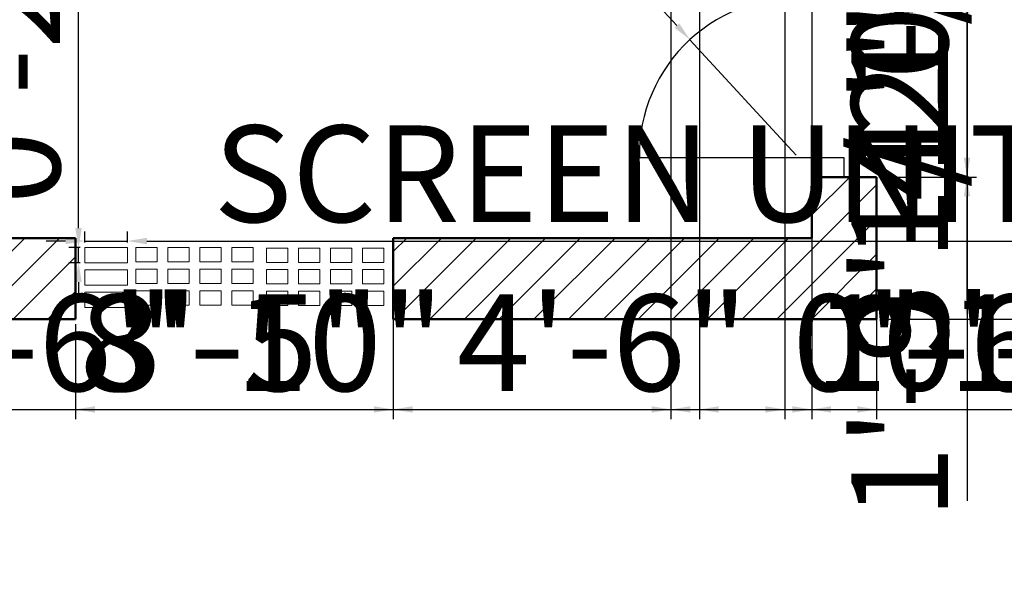
# Model space of a CAD drawing. Units: inches. Extents: x 1545 to 1898, y 1984 to 2198.
# Tile 2 of 4: x 1649 to 1777, y 1984 to 2055. Entities that reach past the tile are written whole.
import ezdxf

# ---------------------------------------------------------------- set-up
doc = ezdxf.new("R2010")
doc.units = ezdxf.units.IN
for name, color, linetype, lineweight in [('A-ANNO-DIMS', 2, 'Continuous', 18), ('A-DOOR', 4, 'Continuous', 25), ('A-WALL', 7, 'Continuous', 50), ('A-WALL-PATT', 252, 'Continuous', 13), ('A-WALL-SCRN', 8, 'Continuous', 18)]:
    doc.layers.add(name, color=color, linetype=linetype, lineweight=lineweight)
doc.styles.get("Standard").update_dxf_attribs({"font": 'arial.ttf'})
doc.dimstyles.new('ISO-25', dxfattribs={"dimtxt": 12.5, "dimasz": 2.5, "dimexe": 1.25, "dimexo": 0.625, "dimtad": 1, "dimdec": 0, "dimlunit": 3, "dimtxsty": 'Standard', "dimcen": 2.5, "dimadec": 0, "dimazin": 0, "dimtfac": 1, "dimtdec": 0, "dimtmove": 0, "dimatfit": 3, "dimfxl": 1, "dimarcsym": 0})

# ---------------------------------------------------------------- blocks, each defined once
blk = doc.blocks.new('*U1')
blk.add_lwpolyline([(-1.38, 0.93), (1.38, 0.93), (1.38, -0.93), (-1.38, -0.93)], close=True)
blk = doc.blocks.new('*U2')
at = {"layer": 'A-WALL-SCRN', "color": 0, "linetype": 'ByBlock', "lineweight": -2, "transparency": 16777216}
for p in [(0, 5.59), (4.14, 5.59), (8.29, 5.59), (12.43, 5.59), (0, 2.8), (4.14, 2.8), (8.29, 2.8), (12.43, 2.8), (0, 0), (4.14, 0), (8.29, 0), (12.43, 0)]:
    blk.add_blockref('*U1', p, dxfattribs=at)
blk = doc.blocks.new('*U3')
blk.add_lwpolyline([(-1.38, 0.93), (1.38, 0.93), (1.38, -0.93), (-1.38, -0.93)], close=True)
blk = doc.blocks.new('*U4')
at = {"layer": 'A-WALL-SCRN', "color": 0, "linetype": 'ByBlock', "lineweight": -2, "transparency": 16777216}
for p in [(0, 5.59), (4.14, 5.59), (8.29, 5.59), (12.43, 5.59), (0, 2.8), (4.14, 2.8), (8.29, 2.8), (12.43, 2.8), (0, 0), (4.14, 0), (8.29, 0), (12.43, 0)]:
    blk.add_blockref('*U3', p, dxfattribs=at)
blk = doc.blocks.new('*D5')
at = {"layer": 'A-ANNO-DIMS', "color": 0, "lineweight": -2, "transparency": 16777216}
for p, q in [((1760.62, 2160.51), (1812.93, 2160.51)), ((1811.68, 2158.01), (1811.68, 2019.01)), ((1760.62, 2016.51), (1812.93, 2016.51))]:
    blk.add_line(p, q, dxfattribs=at)
at = {"layer": 'A-ANNO-DIMS', "color": 0, "transparency": 16777216}
for points in [[(1811.27, 2158.01), (1812.1, 2158.01), (1811.68, 2160.51)], [(1811.27, 2019.01), (1812.1, 2019.01), (1811.68, 2016.51)]]:
    blk.add_solid(points, dxfattribs=at)
at = {"layer": 'Defpoints', "color": 0, "transparency": 16777216}
for p in [(1759.99, 2160.51), (1759.99, 2016.51), (1811.68, 2016.51)]:
    blk.add_point(p, dxfattribs=at)
at = {"layer": 'A-ANNO-DIMS', "color": 0, "transparency": 16777216, "insert": (1804.78, 2088.51), "char_height": 12.5, "attachment_point": 5, "rotation": 90}
blk.add_mtext("12'", dxfattribs=at)
blk = doc.blocks.new('WALL-SCREEN-UNIT')
blk.add_lwpolyline([(0, 1.99), (5.51, 1.99), (5.51, 0), (0, 0)], close=True)
blk = doc.blocks.new('*D7')
at = {"layer": 'A-ANNO-DIMS', "color": 0, "lineweight": -2, "transparency": 16777216}
for p, q in [((1657.6, 2026.41), (1657.6, 2027.87)), ((1663.11, 2026.41), (1663.11, 2027.87)), ((1655.1, 2026.62), (1652.6, 2026.62)), ((1657.6, 2026.62), (1663.11, 2026.62)), ((1665.61, 2026.62), (1897.84, 2026.62))]:
    blk.add_line(p, q, dxfattribs=at)
at = {"layer": 'A-ANNO-DIMS', "color": 0, "transparency": 16777216}
for points in [[(1655.1, 2027.03), (1655.1, 2026.2), (1657.6, 2026.62)], [(1665.61, 2027.03), (1665.61, 2026.2), (1663.11, 2026.62)]]:
    blk.add_solid(points, dxfattribs=at)
at = {"layer": 'Defpoints', "color": 0, "transparency": 16777216}
for p in [(1663.11, 2026.62), (1657.6, 2025.79), (1663.11, 2025.79)]:
    blk.add_point(p, dxfattribs=at)
at = {"layer": 'A-ANNO-DIMS', "color": 0, "transparency": 16777216, "insert": (1782.98, 2033.7), "char_height": 12.5, "attachment_point": 5}
blk.add_mtext('SCREEN UNIT 0\'-5 1/2" TYP.', dxfattribs=at)
blk = doc.blocks.new('*D8')
at = {"layer": 'A-ANNO-DIMS', "color": 0, "lineweight": -2, "transparency": 16777216}
for p, q in [((1656.77, 2028.29), (1656.77, 2108.23)), ((1656.97, 2025.79), (1655.52, 2025.79)), ((1656.77, 2023.8), (1656.77, 2025.79)), ((1656.97, 2023.8), (1655.52, 2023.8)), ((1656.77, 2021.3), (1656.77, 2018.8))]:
    blk.add_line(p, q, dxfattribs=at)
at = {"layer": 'A-ANNO-DIMS', "color": 0, "transparency": 16777216}
for points in [[(1656.35, 2028.29), (1657.19, 2028.29), (1656.77, 2025.79)], [(1656.35, 2021.3), (1657.19, 2021.3), (1656.77, 2023.8)]]:
    blk.add_solid(points, dxfattribs=at)
at = {"layer": 'Defpoints', "color": 0, "transparency": 16777216}
for p in [(1656.77, 2025.79), (1657.6, 2025.79), (1657.6, 2023.8)]:
    blk.add_point(p, dxfattribs=at)
at = {"layer": 'A-ANNO-DIMS', "color": 0, "transparency": 16777216, "insert": (1649.76, 2069.51), "char_height": 12.5, "attachment_point": 5, "rotation": 90}
blk.add_mtext('0\'-2" TYP.', dxfattribs=at)
blk = doc.blocks.new('*D10')
at = {"layer": 'A-ANNO-DIMS', "color": 0, "lineweight": -2, "transparency": 16777216}
for p, q in [((1760.62, 2119.93), (1772.93, 2119.93)), ((1771.68, 2117.43), (1771.68, 2082)), ((1760.62, 2079.5), (1772.93, 2079.5)), ((1771.68, 2079.5), (1771.68, 2013.4))]:
    blk.add_line(p, q, dxfattribs=at)
at = {"layer": 'A-ANNO-DIMS', "color": 0, "transparency": 16777216}
for points in [[(1771.26, 2117.43), (1772.09, 2117.43), (1771.68, 2119.93)], [(1771.26, 2082), (1772.09, 2082), (1771.68, 2079.5)]]:
    blk.add_solid(points, dxfattribs=at)
at = {"layer": 'Defpoints', "color": 0, "transparency": 16777216}
for p in [(1759.99, 2119.93), (1759.99, 2079.5), (1771.68, 2079.5)]:
    blk.add_point(p, dxfattribs=at)
at = {"layer": 'A-ANNO-DIMS', "color": 0, "transparency": 16777216, "insert": (1764.58, 2045.2), "char_height": 12.5, "attachment_point": 5, "rotation": 90}
blk.add_mtext('3\'-4 1/2"', dxfattribs=at)
blk = doc.blocks.new('*D11')
at = {"layer": 'A-ANNO-DIMS', "color": 0, "lineweight": -2, "transparency": 16777216}
for p, q in [((1760.62, 2079.5), (1772.93, 2079.5)), ((1771.68, 2077), (1771.68, 2060.44)), ((1760.62, 2057.94), (1772.93, 2057.94)), ((1771.68, 2057.94), (1771.68, 1993.01))]:
    blk.add_line(p, q, dxfattribs=at)
at = {"layer": 'A-ANNO-DIMS', "color": 0, "transparency": 16777216}
for points in [[(1771.26, 2077), (1772.09, 2077), (1771.68, 2079.5)], [(1771.26, 2060.44), (1772.09, 2060.44), (1771.68, 2057.94)]]:
    blk.add_solid(points, dxfattribs=at)
at = {"layer": 'Defpoints', "color": 0, "transparency": 16777216}
for p in [(1759.99, 2079.5), (1759.99, 2057.94), (1771.68, 2057.94)]:
    blk.add_point(p, dxfattribs=at)
at = {"layer": 'A-ANNO-DIMS', "color": 0, "transparency": 16777216, "insert": (1764.59, 2024.22), "char_height": 12.5, "attachment_point": 5, "rotation": 90}
blk.add_mtext('1\'-9 1/2"', dxfattribs=at)
blk = doc.blocks.new('*D12')
at = {"layer": 'A-ANNO-DIMS', "color": 0, "lineweight": -2, "transparency": 16777216}
for p, q in [((1771.68, 2057.94), (1771.68, 2103.45)), ((1760.62, 2057.94), (1772.93, 2057.94)), ((1771.68, 2037.4), (1771.68, 2055.44)), ((1760.62, 2034.9), (1772.93, 2034.9))]:
    blk.add_line(p, q, dxfattribs=at)
at = {"layer": 'A-ANNO-DIMS', "color": 0, "transparency": 16777216}
for points in [[(1771.26, 2055.44), (1772.09, 2055.44), (1771.68, 2057.94)], [(1771.26, 2037.4), (1772.09, 2037.4), (1771.68, 2034.9)]]:
    blk.add_solid(points, dxfattribs=at)
at = {"layer": 'Defpoints', "color": 0, "transparency": 16777216}
for p in [(1759.99, 2057.94), (1771.68, 2057.94), (1759.99, 2034.9)]:
    blk.add_point(p, dxfattribs=at)
at = {"layer": 'A-ANNO-DIMS', "color": 0, "transparency": 16777216, "insert": (1764.78, 2081.94), "char_height": 12.5, "attachment_point": 5, "rotation": 90}
blk.add_mtext('1\'-11"', dxfattribs=at)
blk = doc.blocks.new('*D13')
at = {"layer": 'A-ANNO-DIMS', "color": 0, "lineweight": -2, "transparency": 16777216}
for p, q in [((1771.68, 2034.9), (1771.68, 2099.83)), ((1760.62, 2034.9), (1772.93, 2034.9)), ((1771.68, 2019.01), (1771.68, 2032.4)), ((1760.62, 2016.51), (1772.93, 2016.51))]:
    blk.add_line(p, q, dxfattribs=at)
at = {"layer": 'A-ANNO-DIMS', "color": 0, "transparency": 16777216}
for points in [[(1771.26, 2032.4), (1772.09, 2032.4), (1771.68, 2034.9)], [(1771.26, 2019.01), (1772.09, 2019.01), (1771.68, 2016.51)]]:
    blk.add_solid(points, dxfattribs=at)
at = {"layer": 'Defpoints', "color": 0, "transparency": 16777216}
for p in [(1759.99, 2034.9), (1771.68, 2034.9), (1759.99, 2016.51)]:
    blk.add_point(p, dxfattribs=at)
at = {"layer": 'A-ANNO-DIMS', "color": 0, "transparency": 16777216, "insert": (1764.59, 2068.62), "char_height": 12.5, "attachment_point": 5, "rotation": 90}
blk.add_mtext('1\'-6 1/2"', dxfattribs=at)
blk = doc.blocks.new('*D19')
at = {"layer": 'A-ANNO-DIMS', "color": 0, "lineweight": -2, "transparency": 16777216}
for p, q in [((1751.61, 2034.28), (1751.61, 2003.57)), ((1759.99, 2034.28), (1759.99, 2003.57)), ((1754.11, 2004.82), (1757.49, 2004.82)), ((1759.99, 2004.82), (1826.1, 2004.82))]:
    blk.add_line(p, q, dxfattribs=at)
at = {"layer": 'A-ANNO-DIMS', "color": 0, "transparency": 16777216}
for points in [[(1754.11, 2005.24), (1754.11, 2004.41), (1751.61, 2004.82)], [(1757.49, 2005.24), (1757.49, 2004.41), (1759.99, 2004.82)]]:
    blk.add_solid(points, dxfattribs=at)
at = {"layer": 'Defpoints', "color": 0, "transparency": 16777216}
for p in [(1751.61, 2034.9), (1759.99, 2034.9), (1759.99, 2004.82)]:
    blk.add_point(p, dxfattribs=at)
at = {"layer": 'A-ANNO-DIMS', "color": 0, "transparency": 16777216, "insert": (1794.29, 2011.91), "char_height": 12.5, "attachment_point": 5}
blk.add_mtext('0\'-8 1/2"', dxfattribs=at)
blk = doc.blocks.new('*D20')
at = {"layer": 'A-ANNO-DIMS', "color": 0, "lineweight": -2, "transparency": 16777216}
for p, q in [((1656.39, 2015.88), (1656.39, 2003.57)), ((1697.47, 2015.88), (1697.47, 2003.57)), ((1658.89, 2004.82), (1694.97, 2004.82))]:
    blk.add_line(p, q, dxfattribs=at)
at = {"layer": 'A-ANNO-DIMS', "color": 0, "transparency": 16777216}
for points in [[(1658.89, 2005.24), (1658.89, 2004.41), (1656.39, 2004.82)], [(1694.97, 2005.24), (1694.97, 2004.41), (1697.47, 2004.82)]]:
    blk.add_solid(points, dxfattribs=at)
at = {"layer": 'Defpoints', "color": 0, "transparency": 16777216}
for p in [(1656.39, 2016.51), (1697.47, 2016.51), (1697.47, 2004.82)]:
    blk.add_point(p, dxfattribs=at)
at = {"layer": 'A-ANNO-DIMS', "color": 0, "transparency": 16777216, "insert": (1676.93, 2011.83), "char_height": 12.5, "attachment_point": 5}
blk.add_mtext('3\'-5"', dxfattribs=at)
blk = doc.blocks.new('*D21')
at = {"layer": 'A-ANNO-DIMS', "color": 0, "lineweight": -2, "transparency": 16777216}
for p, q in [((1697.47, 2026.37), (1697.47, 2003.57)), ((1751.61, 2026.37), (1751.61, 2003.57)), ((1699.97, 2004.82), (1749.11, 2004.82))]:
    blk.add_line(p, q, dxfattribs=at)
at = {"layer": 'A-ANNO-DIMS', "color": 0, "transparency": 16777216}
for points in [[(1699.97, 2005.24), (1699.97, 2004.41), (1697.47, 2004.82)], [(1749.11, 2005.24), (1749.11, 2004.41), (1751.61, 2004.82)]]:
    blk.add_solid(points, dxfattribs=at)
at = {"layer": 'Defpoints', "color": 0, "transparency": 16777216}
for p in [(1697.47, 2027), (1751.61, 2027), (1751.61, 2004.82)]:
    blk.add_point(p, dxfattribs=at)
at = {"layer": 'A-ANNO-DIMS', "color": 0, "transparency": 16777216, "insert": (1724.54, 2011.83), "char_height": 12.5, "attachment_point": 5}
blk.add_mtext('4\'-6"', dxfattribs=at)
blk = doc.blocks.new('*D32')
at = {"layer": 'A-ANNO-DIMS', "color": 0, "lineweight": -2, "transparency": 16777216}
for p, q in [((1734.02, 2122.65), (1772.93, 2122.65)), ((1771.68, 2120.15), (1771.68, 2117.88)), ((1752.23, 2115.38), (1772.93, 2115.38)), ((1771.68, 2115.38), (1771.68, 2049.27))]:
    blk.add_line(p, q, dxfattribs=at)
at = {"layer": 'A-ANNO-DIMS', "color": 0, "transparency": 16777216}
for points in [[(1771.26, 2120.15), (1772.09, 2120.15), (1771.68, 2122.65)], [(1771.26, 2117.88), (1772.09, 2117.88), (1771.68, 2115.38)]]:
    blk.add_solid(points, dxfattribs=at)
at = {"layer": 'Defpoints', "color": 0, "transparency": 16777216}
for p in [(1733.39, 2122.65), (1751.61, 2115.38), (1771.68, 2115.38)]:
    blk.add_point(p, dxfattribs=at)
at = {"layer": 'A-ANNO-DIMS', "color": 0, "transparency": 16777216, "insert": (1764.59, 2081.08), "char_height": 12.5, "attachment_point": 5, "rotation": 90}
blk.add_mtext('0\'-7 1/2"', dxfattribs=at)
blk = doc.blocks.new('*D36')
at = {"layer": 'A-ANNO-DIMS', "color": 0, "lineweight": -2, "transparency": 16777216}
for p, q in [((1600.47, 2063.41), (1600.47, 2003.57)), ((1630.49, 2063.41), (1630.49, 2003.57)), ((1602.97, 2004.82), (1627.99, 2004.82)), ((1630.49, 2004.82), (1667.68, 2004.82))]:
    blk.add_line(p, q, dxfattribs=at)
at = {"layer": 'A-ANNO-DIMS', "color": 0, "transparency": 16777216}
for points in [[(1602.97, 2005.24), (1602.97, 2004.41), (1600.47, 2004.82)], [(1627.99, 2005.24), (1627.99, 2004.41), (1630.49, 2004.82)]]:
    blk.add_solid(points, dxfattribs=at)
at = {"layer": 'Defpoints', "color": 0, "transparency": 16777216}
for p in [(1600.47, 2064.03), (1630.49, 2064.03), (1630.49, 2004.82)]:
    blk.add_point(p, dxfattribs=at)
at = {"layer": 'A-ANNO-DIMS', "color": 0, "transparency": 16777216, "insert": (1650.33, 2011.83), "char_height": 12.5, "attachment_point": 5}
blk.add_mtext('2\'-6"', dxfattribs=at)
blk = doc.blocks.new('*D37')
at = {"layer": 'A-ANNO-DIMS', "color": 0, "lineweight": -2, "transparency": 16777216}
for p, q in [((1733.39, 2065.08), (1733.39, 2003.57)), ((1751.61, 2065.08), (1751.61, 2003.57)), ((1735.89, 2004.82), (1749.11, 2004.82)), ((1751.61, 2004.82), (1787.41, 2004.82))]:
    blk.add_line(p, q, dxfattribs=at)
at = {"layer": 'A-ANNO-DIMS', "color": 0, "transparency": 16777216}
for points in [[(1735.89, 2005.24), (1735.89, 2004.41), (1733.39, 2004.82)], [(1749.11, 2005.24), (1749.11, 2004.41), (1751.61, 2004.82)]]:
    blk.add_solid(points, dxfattribs=at)
at = {"layer": 'Defpoints', "color": 0, "transparency": 16777216}
for p in [(1733.39, 2065.7), (1751.61, 2065.7), (1751.61, 2004.82)]:
    blk.add_point(p, dxfattribs=at)
at = {"layer": 'A-ANNO-DIMS', "color": 0, "transparency": 16777216, "insert": (1770.76, 2011.83), "char_height": 12.5, "attachment_point": 5}
blk.add_mtext('1\'-6"', dxfattribs=at)
blk = doc.blocks.new('*D38')
at = {"layer": 'A-ANNO-DIMS', "color": 0, "lineweight": -2, "transparency": 16777216}
for p, q in [((1627.57, 2127.73), (1627.57, 2003.57)), ((1733.39, 2122.03), (1733.39, 2003.57)), ((1630.07, 2004.82), (1730.89, 2004.82))]:
    blk.add_line(p, q, dxfattribs=at)
at = {"layer": 'A-ANNO-DIMS', "color": 0, "transparency": 16777216}
for points in [[(1630.07, 2005.24), (1630.07, 2004.41), (1627.57, 2004.82)], [(1730.89, 2005.24), (1730.89, 2004.41), (1733.39, 2004.82)]]:
    blk.add_solid(points, dxfattribs=at)
at = {"layer": 'Defpoints', "color": 0, "transparency": 16777216}
for p in [(1627.57, 2128.35), (1733.39, 2122.65), (1733.39, 2004.82)]:
    blk.add_point(p, dxfattribs=at)
at = {"layer": 'A-ANNO-DIMS', "color": 0, "transparency": 16777216, "insert": (1680.48, 2011.83), "char_height": 12.5, "attachment_point": 5}
blk.add_mtext('8\'-10"', dxfattribs=at)
blk = doc.blocks.new('*D41')
at = {"layer": 'A-ANNO-DIMS', "color": 0, "lineweight": -2, "transparency": 16777216}
for p, q in [((1737.08, 2085.23), (1737.08, 2003.57)), ((1748.11, 2085.23), (1748.11, 2003.57)), ((1739.58, 2004.82), (1745.61, 2004.82)), ((1748.11, 2004.82), (1794.8, 2004.82))]:
    blk.add_line(p, q, dxfattribs=at)
at = {"layer": 'A-ANNO-DIMS', "color": 0, "transparency": 16777216}
for points in [[(1739.58, 2005.24), (1739.58, 2004.41), (1737.08, 2004.82)], [(1745.61, 2005.24), (1745.61, 2004.41), (1748.11, 2004.82)]]:
    blk.add_solid(points, dxfattribs=at)
at = {"layer": 'Defpoints', "color": 0, "transparency": 16777216}
for p in [(1737.08, 2085.86), (1748.11, 2085.86), (1748.11, 2004.82)]:
    blk.add_point(p, dxfattribs=at)
at = {"layer": 'A-ANNO-DIMS', "color": 0, "transparency": 16777216, "insert": (1772.71, 2011.83), "char_height": 12.5, "attachment_point": 5}
blk.add_mtext('0\'-11"', dxfattribs=at)
blk = doc.blocks.new('*D43')
at = {"layer": 'A-ANNO-DIMS', "color": 0, "lineweight": -2, "transparency": 16777216}
for p, q in [((1681.27, 2111.93), (1734.16, 2054.51)), ((1749.6, 2037.74), (1735.85, 2052.67))]:
    blk.add_line(p, q, dxfattribs=at)
at = {"layer": 'A-ANNO-DIMS', "color": 0, "transparency": 16777216}
blk.add_solid([(1734.46, 2054.79), (1733.85, 2054.22), (1735.85, 2052.67)], dxfattribs=at)
at = {"layer": 'Defpoints', "color": 0, "transparency": 16777216}
for p in [(1735.85, 2052.67), (1749.6, 2037.74)]:
    blk.add_point(p, dxfattribs=at)
at = {"layer": 'A-ANNO-DIMS', "color": 0, "transparency": 16777216, "insert": (1712.08, 2088.94), "char_height": 12.5, "attachment_point": 5, "rotation": 312.6451}
blk.add_mtext('R1\'-8 1/2"', dxfattribs=at)

msp = doc.modelspace()

# ---------------------------------------------------------------- hatches: boundary and pattern name
at = {"layer": 'A-WALL-PATT'}
h = msp.add_hatch(dxfattribs=at)
h.set_pattern_fill('ANSI31', color=256)
h.paths.add_polyline_path([(1656.39, 2027), (1591.27, 2027), (1591.27, 2016.51), (1604.23, 2016.51), (1656.39, 2016.51)])
h.paths.add_polyline_path([(1759.99, 2034.9), (1751.61, 2034.9), (1751.61, 2027), (1697.47, 2027), (1697.47, 2016.51), (1759.99, 2016.51)])

# ---------------------------------------------------------------- linework, layer by layer
at = {"layer": 'A-DOOR'}
for p, q in [((1755.8, 2037.4), (1729.31, 2037.4)), ((1755.8, 2034.9), (1755.8, 2037.4))]:
    msp.add_line(p, q, dxfattribs=at)
msp.add_arc((1749.6, 2037.74), 20.3, 84.3172, 180.9706, dxfattribs=at)
at = {"layer": 'A-WALL'}
for p, q in [((1751.61, 2034.9), (1759.99, 2034.9)), ((1751.61, 2034.9), (1751.61, 2027)), ((1759.99, 2034.9), (1759.99, 2016.51)), ((1656.39, 2027), (1591.27, 2027)), ((1656.39, 2027), (1656.39, 2016.51)), ((1751.61, 2027), (1697.47, 2027)), ((1697.47, 2016.51), (1697.47, 2027)), ((1656.39, 2016.51), (1604.23, 2016.51)), ((1759.99, 2016.51), (1697.47, 2016.51))]:
    msp.add_line(p, q, dxfattribs=at)

# ---------------------------------------------------------------- block references
at = {"layer": 'A-WALL-SCRN'}
for name, p in [('WALL-SCREEN-UNIT', (1657.6, 2023.8)), ('*U4', (1665.55, 2019.26)), ('*U2', (1682.45, 2019.19)), ('WALL-SCREEN-UNIT', (1657.6, 2020.9)), ('WALL-SCREEN-UNIT', (1657.6, 2018.03))]:
    msp.add_blockref(name, p, dxfattribs=at)

# ---------------------------------------------------------------- dimensions: what is measured, and where the dimension line sits
at = {"layer": 'A-ANNO-DIMS'}
for base, p1, p2, override, picture, middle in [((1811.68, 2016.51), (1759.99, 2160.51), (1759.99, 2016.51), {"dimclrd": 0, "dimclre": 0, "dimclrt": 0}, '*D5', (1804.78, 2088.51)), ((1771.68, 2115.38), (1733.39, 2122.65), (1751.61, 2115.38), {"dimdec": 1, "dimlfac": 1, "dimrnd": 0, "dimzin": 1, "dimdsep": 46, "dimlunit": 4, "dimfrac": 2}, '*D32', (1764.59, 2081.08)), ((1771.68, 2079.5), (1759.99, 2119.93), (1759.99, 2079.5), {"dimdec": 1, "dimlfac": 1, "dimrnd": 0, "dimzin": 1, "dimdsep": 46, "dimlunit": 4, "dimfrac": 2}, '*D10', (1764.58, 2045.2)), ((1771.68, 2057.94), (1759.99, 2034.9), (1759.99, 2057.94), {"dimdec": 1, "dimlfac": 1, "dimrnd": 0, "dimzin": 1, "dimdsep": 46, "dimlunit": 4, "dimfrac": 2}, '*D12', (1764.78, 2081.94)), ((1771.68, 2034.9), (1759.99, 2016.51), (1759.99, 2034.9), {"dimdec": 1, "dimlfac": 1, "dimrnd": 0, "dimzin": 1, "dimdsep": 46, "dimlunit": 4, "dimfrac": 2}, '*D13', (1764.59, 2068.62)), ((1771.68, 2057.94), (1759.99, 2079.5), (1759.99, 2057.94), {"dimdec": 1, "dimlfac": 1, "dimrnd": 0, "dimzin": 1, "dimdsep": 46, "dimlunit": 4, "dimfrac": 2}, '*D11', (1764.59, 2024.22))]:
    dim = msp.add_linear_dim(base=base, p1=p1, p2=p2, angle=90, dimstyle='ISO-25', override=override, dxfattribs=at)
    dim.commit()
    dim.dimension.update_dxf_attribs({"geometry": picture, "text_midpoint": middle})
for base, p1, p2, picture, middle in [((1733.39, 2004.82), (1627.57, 2128.35), (1733.39, 2122.65), '*D38', (1680.48, 2011.83)), ((1748.11, 2004.82), (1737.08, 2085.86), (1748.11, 2085.86), '*D41', (1772.71, 2011.83)), ((1751.61, 2004.82), (1733.39, 2065.7), (1751.61, 2065.7), '*D37', (1770.76, 2011.83)), ((1630.49, 2004.82), (1600.47, 2064.03), (1630.49, 2064.03), '*D36', (1650.33, 2011.83)), ((1759.99, 2004.82), (1751.61, 2034.9), (1759.99, 2034.9), '*D19', (1794.29, 2011.91)), ((1751.61, 2004.82), (1697.47, 2027), (1751.61, 2027), '*D21', (1724.54, 2011.83)), ((1697.47, 2004.82), (1656.39, 2016.51), (1697.47, 2016.51), '*D20', (1676.93, 2011.83))]:
    dim = msp.add_linear_dim(base=base, p1=p1, p2=p2, dimstyle='ISO-25', override={"dimdec": 1, "dimlfac": 1, "dimrnd": 0, "dimzin": 1, "dimdsep": 46, "dimlunit": 4, "dimfrac": 2}, dxfattribs=at)
    dim.commit()
    dim.dimension.update_dxf_attribs({"geometry": picture, "text_midpoint": middle})
dim = msp.add_radius_dim(center=(1749.6, 2037.74), mpoint=(1735.85, 2052.67), dimstyle='ISO-25', override={"dimdec": 1, "dimlfac": 1, "dimrnd": 0, "dimzin": 1, "dimdsep": 46, "dimlunit": 4, "dimfrac": 2}, dxfattribs=at)
dim.commit()
dim.dimension.update_dxf_attribs({"geometry": '*D43', "text_midpoint": (1712.08, 2088.94)})
dim = msp.add_linear_dim(base=(1656.77, 2025.79), p1=(1657.6, 2023.8), p2=(1657.6, 2025.79), angle=90, text='<> TYP.', dimstyle='ISO-25', override={"dimdec": 1, "dimlfac": 1, "dimrnd": 0, "dimzin": 1, "dimdsep": 46, "dimlunit": 4, "dimfrac": 2}, dxfattribs=at)
dim.commit()
dim.dimension.update_dxf_attribs({"geometry": '*D8', "text_midpoint": (1649.76, 2069.51)})
dim = msp.add_linear_dim(base=(1663.11, 2026.62), p1=(1657.6, 2025.79), p2=(1663.11, 2025.79), text='SCREEN UNIT <> TYP.', dimstyle='ISO-25', override={"dimdec": 1, "dimlfac": 1, "dimrnd": 0, "dimzin": 1, "dimdsep": 46, "dimlunit": 4, "dimfrac": 2}, dxfattribs=at)
dim.commit()
dim.dimension.update_dxf_attribs({"geometry": '*D7', "text_midpoint": (1782.98, 2033.7)})

doc.saveas('drawing.dxf')
